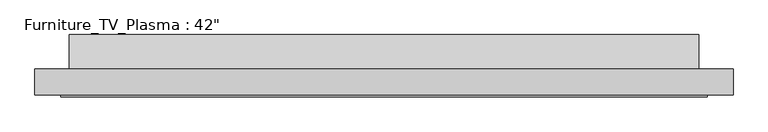
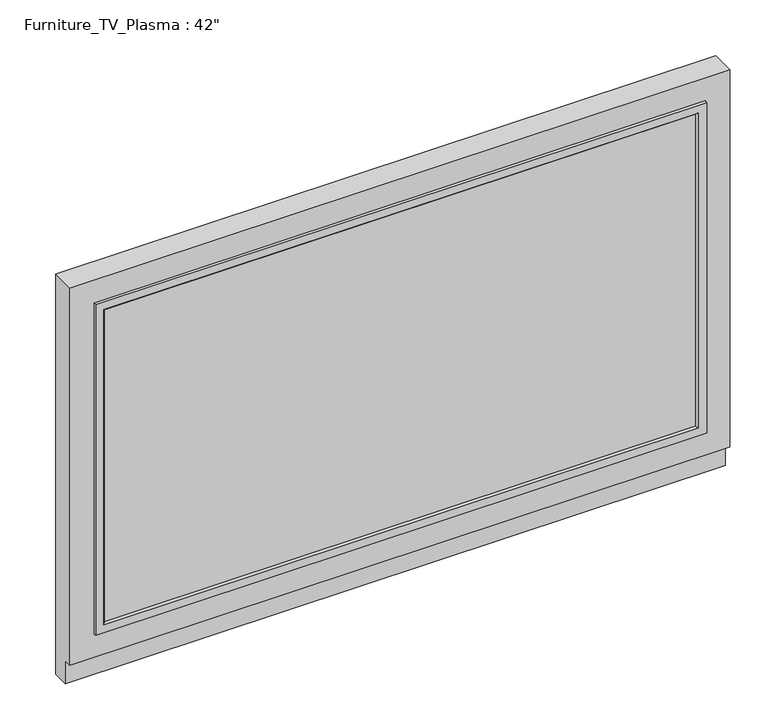
"""IFC4 building model written with IfcOpenShell, lengths in millimetres: furniture geometry."""

from ifc_helpers import new_model, si_unit, frame, origin, place, context, project, spatial, polyline, outline, extrude, faceted_brep, source, transform, mapped, element, save


def furniture_0b97a49d(model_context):
    return source(origin(), model_context, "Body", "SolidModel", [
        faceted_brep([(571.5, -50.8, 660.4), (-457.2, -50.8, 660.4), (-457.2, -88.9, 660.4), (571.5, -88.9, 660.4), (-457.2, -50.8, 0.0), (571.5, -50.8, 0.0), (571.5, -76.2, 0.0), (-457.2, -76.2, 0.0), (-457.2, -76.2, 38.1), (-457.2, -88.9, 38.1), (571.5, -88.9, 38.1), (533.4, -88.9, 622.3), (533.4, -88.9, 76.2), (-419.1, -88.9, 76.2), (-419.1, -88.9, 622.3), (571.5, -76.2, 38.1), (533.4, -74.1720413, 622.3), (-419.1, -74.1720413, 622.3), (-419.1, -74.1720413, 76.2), (533.4, -74.1720413, 76.2)], [[[0, 1, 2, 3]], [[4, 5, 6, 7]], [[1, 0, 5, 4]], [[2, 1, 4, 7, 8, 9]], [[3, 2, 9, 10], [11, 12, 13, 14]], [[0, 3, 10, 15, 6, 5]], [[16, 17, 18, 19]], [[16, 19, 12, 11]], [[19, 18, 13, 12]], [[18, 17, 14, 13]], [[17, 16, 11, 14]], [[15, 8, 7, 6]], [[8, 15, 10, 9]]]),
        extrude(outline(polyline([(520.7, -88.9), (-406.4, -88.9), (-406.4, -74.1720413), (520.7, -74.1720413), (520.7, -88.9)])), frame((0.0, 0.0, 88.9), z_axis=(0.0, 0.0, 1.0), x_axis=(1.0, 0.0, 0.0)), (0.0, 0.0, 1.0), 520.7),
        extrude(outline(polyline([(0.0, 574.8688953), (0.0, 38.1), (-50.8, 38.1), (-50.8, 609.6), (0.0, 574.8688953)])), frame((-406.4, 0.0, 0.0), z_axis=(1.0, 0.0, 0.0), x_axis=(0.0, 1.0, 0.0)), (0.0, 0.0, 1.0), 927.1),
        faceted_brep([(517.525, -88.9, 92.075), (520.7, -92.075, 88.9), (520.7, -92.075, 608.80625), (517.525, -88.9, 605.63125), (520.7, -74.1720413, 88.9), (520.7, -88.9, 88.9), (520.7, -88.9, 608.80625), (520.7, -74.1720413, 608.80625), (533.4, -92.075, 76.2), (533.4, -74.1720413, 76.2), (533.4, -74.1720413, 621.50625), (533.4, -92.075, 621.50625), (-406.4, -92.075, 608.80625), (-403.225, -88.9, 605.63125), (-406.4, -88.9, 608.80625), (-406.4, -74.1720413, 608.80625), (-419.1, -74.1720413, 621.50625), (-419.1, -92.075, 621.50625), (-406.4, -92.075, 88.9), (-403.225, -88.9, 92.075), (-406.4, -88.9, 88.9), (-406.4, -74.1720413, 88.9), (-419.1, -74.1720413, 76.2), (-419.1, -92.075, 76.2)], [[[0, 1, 2, 3]], [[4, 5, 6, 7]], [[8, 9, 10, 11]], [[3, 2, 12, 13]], [[7, 6, 14, 15]], [[11, 10, 16, 17]], [[13, 12, 18, 19]], [[15, 14, 20, 21]], [[17, 16, 22, 23]], [[11, 17, 23, 8], [1, 18, 12, 2]], [[19, 18, 1, 0]], [[5, 20, 14, 6], [3, 13, 19, 0]], [[21, 20, 5, 4]], [[9, 22, 16, 10], [7, 15, 21, 4]], [[23, 22, 9, 8]]]),
    ])


if __name__ == "__main__":
    model = new_model("IFC4")
    model_context = context("Model", 3, world=origin())
    ifc_project = project(units=[si_unit("LENGTHUNIT", "METRE", prefix="MILLI")], contexts=[model_context])
    site = spatial("IfcSite", under=ifc_project)
    building = spatial("IfcBuilding", under=site)
    placement = place(None, origin())
    furniture_shape = furniture_0b97a49d(model_context)
    element("IfcFurniture", 1, ObjectType="Furniture_TV_Plasma : 42\"", at=placement, inside=building, context=model_context, shape_type="MappedRepresentation", body=[
        mapped(furniture_shape, transform((0.0, 0.0, 0.0), x_axis=(1.0, 0.0, 0.0), y_axis=(0.0, 1.0, 0.0), z_axis=(0.0, 0.0, 1.0))),
    ])
    save(model, "model.ifc")

# Revit data of these elements
# Type "Furniture_TV_Plasma : 42\""
#   Keynote = "N"
#   Assembly Code = "E2020200"
#   Depth = 0' - 3 1/2"
#   Height = 2' - 2"
#   Width = 3' - 4 1/2"
#   Material Cabinet = Plastic - Gray
#   Default Elevation = 0
# Element 1 (IfcFurniture, "Furniture_TV_Plasma : 42\"")
#   Materials on its faces: "Plastic - Black", "Plastic - Gray", "Glass"
# Materials
#   "Plastic - Gray": class "Plastic", colour RGB 134 134 134, transparency 0
#   "Plastic - Black": class "Plastic", colour RGB 0 0 0, transparency 0
#   "Glass": class "Glass", colour RGB 0 128 192, transparency 0.75, Description = "Soda Lime Glass", Cost = 0
